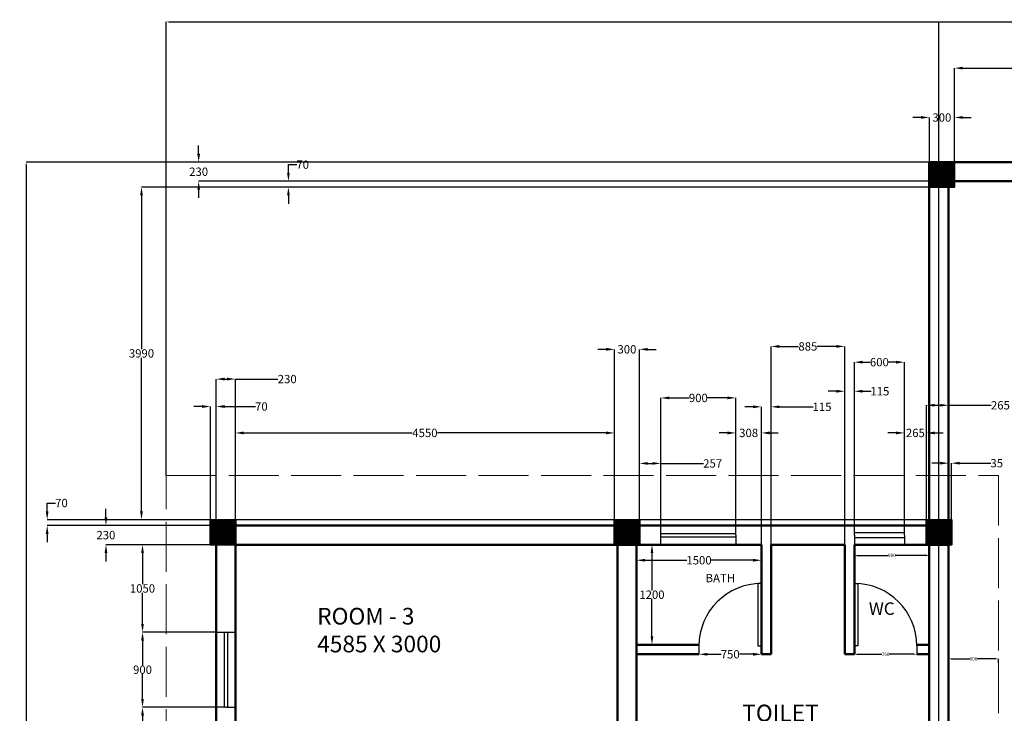
# Model space of a CAD drawing. Units: millimetres. Extents: x -17156 to 39375, y -45872 to -24892.
# Tile 3 of 12: x -17156 to -5337, y -33861 to -25539. Entities that reach past the tile are written whole.
import ezdxf

# ---------------------------------------------------------------- set-up
doc = ezdxf.new("R2010")
doc.units = ezdxf.units.MM
doc.header["$MEASUREMENT"] = 0
doc.linetypes.add('ACAD_ISO02W100', pattern=[15, 12, -3])
for name, color, linetype, lineweight in [('A-ANNO-DIMS', 2, 'Continuous', 18), ('A-AREA-IDEN', 4, 'Continuous', 25), ('A-COLS', 7, 'Continuous', 40), ('A-ROOF-OVHD', 8, 'ACAD_ISO02W100', 18), ('DOORS', 6, 'Continuous', 25), ('WALLS', 5, 'Continuous', 50), ('WINDOW', 240, 'Continuous', 25)]:
    doc.layers.add(name, color=color, linetype=linetype, lineweight=lineweight)
doc.styles.get("Standard").update_dxf_attribs({"font": 'arial.ttf'})
doc.dimstyles.get("Standard").update_dxf_attribs({"dimtxt": 40, "dimasz": 30.18, "dimexe": 0, "dimexo": 0.0625, "dimgap": 0.09, "dimtad": 0, "dimtih": 1, "dimtoh": 1, "dimdec": 0, "dimzin": 0, "dimdsep": 46, "dimtxsty": 'Standard', "dimcen": 0.09, "dimadec": 0, "dimazin": 0, "dimtfac": 1, "dimtdec": 0, "dimtofl": 0, "dimtmove": 0, "dimatfit": 3, "dimfxl": 1, "dimtolj": 1, "dimtzin": 0, "dimarcsym": 0})

# ---------------------------------------------------------------- blocks, each defined once
blk = doc.blocks.new('*U3')
for p, q in [((-750, 0), (-750, -100)), ((0, 0), (0, -100))]:
    blk.add_line(p, q)
blk.add_lwpolyline([(0, 0), (0, 750), (-43.75, 750), (-43.75, 0)], close=True)
blk.add_arc((0, 0), 750, 90, 180)
blk = doc.blocks.new('*U5')
for p, q in [((0, 0), (0, -100)), ((750, 0), (750, -100))]:
    blk.add_line(p, q)
blk.add_lwpolyline([(0, 0), (0, 750), (43.75, 750), (43.75, 0)], close=True)
blk.add_arc((0, 0), 750, 0, 90)
blk = doc.blocks.new('*D23')
at = {"layer": 'A-ANNO-DIMS', "color": 0, "lineweight": -2, "transparency": 16777216}
for p, q in [((-14797, -33788), (-15682, -33788)), ((-15682, -33888), (-15682, -34262)), ((-15682, -34738), (-15682, -34364)), ((-14867, -34838), (-15682, -34838))]:
    blk.add_line(p, q, dxfattribs=at)
at = {"layer": 'A-ANNO-DIMS', "color": 0, "lineweight": 100, "transparency": 16777216}
for points in [[(-15698, -33888), (-15665, -33888), (-15682, -33788)], [(-15698, -34738), (-15665, -34738), (-15682, -34838)]]:
    blk.add_solid(points, dxfattribs=at)
at = {"layer": 'Defpoints', "color": 0, "lineweight": 100, "transparency": 16777216}
for p in [(-15682, -33788), (-14797, -33788), (-14867, -34838)]:
    blk.add_point(p, dxfattribs=at)
at = {"layer": 'A-ANNO-DIMS', "color": 0, "transparency": 16777216, "insert": (-15682, -34313), "char_height": 100, "attachment_point": 5}
blk.add_mtext('\\A1;1050', dxfattribs=at)
blk = doc.blocks.new('*D24')
at = {"layer": 'A-ANNO-DIMS', "color": 0, "lineweight": -2, "transparency": 16777216}
for p, q in [((-14797, -32888), (-15682, -32888)), ((-15682, -32988), (-15682, -33287)), ((-15682, -33688), (-15682, -33389)), ((-14797, -33788), (-15682, -33788))]:
    blk.add_line(p, q, dxfattribs=at)
at = {"layer": 'A-ANNO-DIMS', "color": 0, "lineweight": 100, "transparency": 16777216}
for points in [[(-15698, -32988), (-15665, -32988), (-15682, -32888)], [(-15698, -33688), (-15665, -33688), (-15682, -33788)]]:
    blk.add_solid(points, dxfattribs=at)
at = {"layer": 'Defpoints', "color": 0, "lineweight": 100, "transparency": 16777216}
for p in [(-15682, -32888), (-14797, -32888), (-14797, -33788)]:
    blk.add_point(p, dxfattribs=at)
at = {"layer": 'A-ANNO-DIMS', "color": 0, "transparency": 16777216, "insert": (-15682, -33338), "char_height": 100, "attachment_point": 5}
blk.add_mtext('\\A1;900', dxfattribs=at)
blk = doc.blocks.new('*D25')
at = {"layer": 'A-ANNO-DIMS', "color": 0, "lineweight": -2, "transparency": 16777216}
for p, q in [((-14867, -31838), (-15682, -31838)), ((-15682, -31938), (-15682, -32312)), ((-15682, -32788), (-15682, -32414)), ((-14797, -32888), (-15682, -32888))]:
    blk.add_line(p, q, dxfattribs=at)
at = {"layer": 'A-ANNO-DIMS', "color": 0, "lineweight": 100, "transparency": 16777216}
for points in [[(-15698, -31938), (-15665, -31938), (-15682, -31838)], [(-15698, -32788), (-15665, -32788), (-15682, -32888)]]:
    blk.add_solid(points, dxfattribs=at)
at = {"layer": 'Defpoints', "color": 0, "lineweight": 100, "transparency": 16777216}
for p in [(-15682, -31838), (-14867, -31838), (-14797, -32888)]:
    blk.add_point(p, dxfattribs=at)
at = {"layer": 'A-ANNO-DIMS', "color": 0, "transparency": 16777216, "insert": (-15682, -32363), "char_height": 100, "attachment_point": 5}
blk.add_mtext('\\A1;1050', dxfattribs=at)
blk = doc.blocks.new('*D26')
at = {"layer": 'A-ANNO-DIMS', "color": 0, "lineweight": -2, "transparency": 16777216}
for p, q in [((-16121, -31508), (-16121, -31408)), ((-14797, -31608), (-16121, -31608)), ((-14867, -31838), (-16121, -31838)), ((-16121, -31938), (-16121, -32038))]:
    blk.add_line(p, q, dxfattribs=at)
at = {"layer": 'A-ANNO-DIMS', "color": 0, "lineweight": 100, "transparency": 16777216}
for points in [[(-16137, -31508), (-16104, -31508), (-16121, -31608)], [(-16137, -31938), (-16104, -31938), (-16121, -31838)]]:
    blk.add_solid(points, dxfattribs=at)
at = {"layer": 'Defpoints', "color": 0, "lineweight": 100, "transparency": 16777216}
for p in [(-16121, -31608), (-14797, -31608), (-14867, -31838)]:
    blk.add_point(p, dxfattribs=at)
at = {"layer": 'A-ANNO-DIMS', "color": 0, "transparency": 16777216, "insert": (-16121, -31723), "char_height": 100, "attachment_point": 5}
blk.add_mtext('\\A1;230', dxfattribs=at)
blk = doc.blocks.new('*D27')
at = {"layer": 'A-ANNO-DIMS', "color": 0, "lineweight": -2, "transparency": 16777216}
for p, q in [((-16826, -31438), (-16826, -31338)), ((-16826, -31338), (-16726, -31338)), ((-14867, -31538), (-16826, -31538)), ((-14797, -31608), (-16826, -31608)), ((-16826, -31708), (-16826, -31808))]:
    blk.add_line(p, q, dxfattribs=at)
at = {"layer": 'A-ANNO-DIMS', "color": 0, "lineweight": 100, "transparency": 16777216}
for points in [[(-16843, -31438), (-16810, -31438), (-16826, -31538)], [(-16843, -31708), (-16810, -31708), (-16826, -31608)]]:
    blk.add_solid(points, dxfattribs=at)
at = {"layer": 'Defpoints', "color": 0, "lineweight": 100, "transparency": 16777216}
for p in [(-16826, -31538), (-14867, -31538), (-14797, -31608)]:
    blk.add_point(p, dxfattribs=at)
at = {"layer": 'A-ANNO-DIMS', "color": 0, "transparency": 16777216, "insert": (-16655, -31338), "char_height": 100, "attachment_point": 5}
blk.add_mtext('\\A1;70', dxfattribs=at)
blk = doc.blocks.new('*D28')
at = {"layer": 'A-ANNO-DIMS', "color": 0, "lineweight": -2, "transparency": 16777216}
for p, q in [((-6237, -27548), (-15694, -27548)), ((-15694, -27648), (-15694, -29492)), ((-15694, -31438), (-15694, -29594)), ((-6272, -31538), (-15694, -31538))]:
    blk.add_line(p, q, dxfattribs=at)
at = {"layer": 'A-ANNO-DIMS', "color": 0, "lineweight": 100, "transparency": 16777216}
for points in [[(-15711, -27648), (-15677, -27648), (-15694, -27548)], [(-15711, -31438), (-15677, -31438), (-15694, -31538)]]:
    blk.add_solid(points, dxfattribs=at)
at = {"layer": 'Defpoints', "color": 0, "lineweight": 100, "transparency": 16777216}
for p in [(-15694, -27548), (-6237, -27548), (-6272, -31538)]:
    blk.add_point(p, dxfattribs=at)
at = {"layer": 'A-ANNO-DIMS', "color": 0, "transparency": 16777216, "insert": (-15694, -29543), "char_height": 100, "attachment_point": 5}
blk.add_mtext('\\A1;3990', dxfattribs=at)
blk = doc.blocks.new('*D29')
at = {"layer": 'A-ANNO-DIMS', "color": 0, "lineweight": -2, "transparency": 16777216}
for p, q in [((-13930, -27378), (-13930, -27278)), ((-13930, -27278), (-13830, -27278)), ((-6237, -27478), (-13930, -27478)), ((-6237, -27548), (-13930, -27548)), ((-13930, -27648), (-13930, -27748))]:
    blk.add_line(p, q, dxfattribs=at)
at = {"layer": 'A-ANNO-DIMS', "color": 0, "lineweight": 100, "transparency": 16777216}
for points in [[(-13947, -27378), (-13914, -27378), (-13930, -27478)], [(-13947, -27648), (-13914, -27648), (-13930, -27548)]]:
    blk.add_solid(points, dxfattribs=at)
at = {"layer": 'Defpoints', "color": 0, "lineweight": 100, "transparency": 16777216}
for p in [(-13930, -27478), (-6237, -27478), (-6237, -27548)]:
    blk.add_point(p, dxfattribs=at)
at = {"layer": 'A-ANNO-DIMS', "color": 0, "transparency": 16777216, "insert": (-13759, -27278), "char_height": 100, "attachment_point": 5}
blk.add_mtext('\\A1;70', dxfattribs=at)
blk = doc.blocks.new('*D30')
at = {"layer": 'A-ANNO-DIMS', "color": 0, "lineweight": -2, "transparency": 16777216}
for p, q in [((-15008, -27148), (-15008, -27048)), ((-6237, -27248), (-15008, -27248)), ((-6237, -27478), (-15008, -27478)), ((-15008, -27578), (-15008, -27678))]:
    blk.add_line(p, q, dxfattribs=at)
at = {"layer": 'A-ANNO-DIMS', "color": 0, "lineweight": 100, "transparency": 16777216}
for points in [[(-15024, -27148), (-14991, -27148), (-15008, -27248)], [(-15024, -27578), (-14991, -27578), (-15008, -27478)]]:
    blk.add_solid(points, dxfattribs=at)
at = {"layer": 'Defpoints', "color": 0, "lineweight": 100, "transparency": 16777216}
for p in [(-15008, -27248), (-6237, -27248), (-6237, -27478)]:
    blk.add_point(p, dxfattribs=at)
at = {"layer": 'A-ANNO-DIMS', "color": 0, "transparency": 16777216, "insert": (-15008, -27363), "char_height": 100, "attachment_point": 5}
blk.add_mtext('\\A1;230', dxfattribs=at)
blk = doc.blocks.new('*D52')
at = {"layer": 'A-ANNO-DIMS', "color": 0, "lineweight": -2, "transparency": 16777216}
for p, q in [((-14967, -30180), (-15067, -30180)), ((-14867, -31538), (-14867, -30180)), ((-14797, -31608), (-14797, -30180)), ((-14697, -30180), (-14326, -30180))]:
    blk.add_line(p, q, dxfattribs=at)
at = {"layer": 'A-ANNO-DIMS', "color": 0, "lineweight": 100, "transparency": 16777216}
for points in [[(-14967, -30163), (-14967, -30197), (-14867, -30180)], [(-14697, -30163), (-14697, -30197), (-14797, -30180)]]:
    blk.add_solid(points, dxfattribs=at)
at = {"layer": 'Defpoints', "color": 0, "lineweight": 100, "transparency": 16777216}
for p in [(-14797, -30180), (-14867, -31538), (-14797, -31608)]:
    blk.add_point(p, dxfattribs=at)
at = {"layer": 'A-ANNO-DIMS', "color": 0, "transparency": 16777216, "insert": (-14255, -30180), "char_height": 100, "attachment_point": 5}
blk.add_mtext('\\A1;70', dxfattribs=at)
blk = doc.blocks.new('*D53')
at = {"layer": 'A-ANNO-DIMS', "color": 0, "lineweight": -2, "transparency": 16777216}
for p, q in [((-14797, -31608), (-14797, -29851)), ((-14697, -29851), (-14667, -29851)), ((-14567, -31538), (-14567, -29851)), ((-14567, -29851), (-14056, -29851))]:
    blk.add_line(p, q, dxfattribs=at)
at = {"layer": 'A-ANNO-DIMS', "color": 0, "lineweight": 100, "transparency": 16777216}
for points in [[(-14697, -29834), (-14697, -29867), (-14797, -29851)], [(-14667, -29834), (-14667, -29867), (-14567, -29851)]]:
    blk.add_solid(points, dxfattribs=at)
at = {"layer": 'Defpoints', "color": 0, "lineweight": 100, "transparency": 16777216}
for p in [(-14567, -29851), (-14567, -31538), (-14797, -31608)]:
    blk.add_point(p, dxfattribs=at)
at = {"layer": 'A-ANNO-DIMS', "color": 0, "transparency": 16777216, "insert": (-13945, -29851), "char_height": 100, "attachment_point": 5}
blk.add_mtext('\\A1;230', dxfattribs=at)
blk = doc.blocks.new('*D54')
at = {"layer": 'A-ANNO-DIMS', "color": 0, "lineweight": -2, "transparency": 16777216}
for p, q in [((-14567, -31538), (-14567, -30497)), ((-14467, -30497), (-12444, -30497)), ((-10117, -30497), (-12141, -30497)), ((-10017, -31538), (-10017, -30497))]:
    blk.add_line(p, q, dxfattribs=at)
at = {"layer": 'A-ANNO-DIMS', "color": 0, "lineweight": 100, "transparency": 16777216}
for points in [[(-14467, -30480), (-14467, -30514), (-14567, -30497)], [(-10117, -30480), (-10117, -30514), (-10017, -30497)]]:
    blk.add_solid(points, dxfattribs=at)
at = {"layer": 'Defpoints', "color": 0, "lineweight": 100, "transparency": 16777216}
for p in [(-10017, -30497), (-14567, -31538), (-10017, -31538)]:
    blk.add_point(p, dxfattribs=at)
at = {"layer": 'A-ANNO-DIMS', "color": 0, "transparency": 16777216, "insert": (-12292, -30497), "char_height": 100, "attachment_point": 5}
blk.add_mtext('\\A1;4550', dxfattribs=at)
blk = doc.blocks.new('*D55')
at = {"layer": 'A-ANNO-DIMS', "color": 0, "lineweight": -2, "transparency": 16777216}
for p, q in [((-10117, -29494), (-10217, -29494)), ((-10017, -31538), (-10017, -29494)), ((-9717, -31538), (-9717, -29494)), ((-9617, -29494), (-9517, -29494))]:
    blk.add_line(p, q, dxfattribs=at)
at = {"layer": 'A-ANNO-DIMS', "color": 0, "lineweight": 100, "transparency": 16777216}
for points in [[(-10117, -29477), (-10117, -29511), (-10017, -29494)], [(-9617, -29477), (-9617, -29511), (-9717, -29494)]]:
    blk.add_solid(points, dxfattribs=at)
at = {"layer": 'Defpoints', "color": 0, "lineweight": 100, "transparency": 16777216}
for p in [(-9717, -29494), (-10017, -31538), (-9717, -31538)]:
    blk.add_point(p, dxfattribs=at)
at = {"layer": 'A-ANNO-DIMS', "color": 0, "transparency": 16777216, "insert": (-9867, -29494), "char_height": 100, "attachment_point": 5}
blk.add_mtext('\\A1;300', dxfattribs=at)
blk = doc.blocks.new('*D56')
at = {"layer": 'A-ANNO-DIMS', "color": 0, "lineweight": -2, "transparency": 16777216}
for p, q in [((-9717, -31538), (-9717, -30863)), ((-9617, -30863), (-9560, -30863)), ((-9460, -31608), (-9460, -30863)), ((-9460, -30863), (-8949, -30863))]:
    blk.add_line(p, q, dxfattribs=at)
at = {"layer": 'A-ANNO-DIMS', "color": 0, "lineweight": 100, "transparency": 16777216}
for points in [[(-9617, -30846), (-9617, -30879), (-9717, -30863)], [(-9560, -30846), (-9560, -30879), (-9460, -30863)]]:
    blk.add_solid(points, dxfattribs=at)
at = {"layer": 'Defpoints', "color": 0, "lineweight": 100, "transparency": 16777216}
for p in [(-9460, -30863), (-9717, -31538), (-9460, -31608)]:
    blk.add_point(p, dxfattribs=at)
at = {"layer": 'A-ANNO-DIMS', "color": 0, "transparency": 16777216, "insert": (-8838, -30863), "char_height": 100, "attachment_point": 5}
blk.add_mtext('\\A1;257', dxfattribs=at)
blk = doc.blocks.new('*D57')
at = {"layer": 'A-ANNO-DIMS', "color": 0, "lineweight": -2, "transparency": 16777216}
for p, q in [((-9460, -31608), (-9460, -30077)), ((-9360, -30077), (-9121, -30077)), ((-8660, -30077), (-8900, -30077)), ((-8560, -31608), (-8560, -30077))]:
    blk.add_line(p, q, dxfattribs=at)
at = {"layer": 'A-ANNO-DIMS', "color": 0, "lineweight": 100, "transparency": 16777216}
for points in [[(-9360, -30060), (-9360, -30093), (-9460, -30077)], [(-8660, -30060), (-8660, -30093), (-8560, -30077)]]:
    blk.add_solid(points, dxfattribs=at)
at = {"layer": 'Defpoints', "color": 0, "lineweight": 100, "transparency": 16777216}
for p in [(-8560, -30077), (-9460, -31608), (-8560, -31608)]:
    blk.add_point(p, dxfattribs=at)
at = {"layer": 'A-ANNO-DIMS', "color": 0, "transparency": 16777216, "insert": (-9010, -30077), "char_height": 100, "attachment_point": 5}
blk.add_mtext('\\A1;900', dxfattribs=at)
blk = doc.blocks.new('*D58')
at = {"layer": 'A-ANNO-DIMS', "color": 0, "lineweight": -2, "transparency": 16777216}
for p, q in [((-8660, -30497), (-8760, -30497)), ((-8560, -31608), (-8560, -30497)), ((-8252, -31838), (-8252, -30497)), ((-8152, -30497), (-8052, -30497))]:
    blk.add_line(p, q, dxfattribs=at)
at = {"layer": 'A-ANNO-DIMS', "color": 0, "lineweight": 100, "transparency": 16777216}
for points in [[(-8660, -30480), (-8660, -30514), (-8560, -30497)], [(-8152, -30480), (-8152, -30514), (-8252, -30497)]]:
    blk.add_solid(points, dxfattribs=at)
at = {"layer": 'Defpoints', "color": 0, "lineweight": 100, "transparency": 16777216}
for p in [(-8252, -30497), (-8560, -31608), (-8252, -31838)]:
    blk.add_point(p, dxfattribs=at)
at = {"layer": 'A-ANNO-DIMS', "color": 0, "transparency": 16777216, "insert": (-8406, -30497), "char_height": 100, "attachment_point": 5}
blk.add_mtext('\\A1;308', dxfattribs=at)
blk = doc.blocks.new('*D59')
at = {"layer": 'A-ANNO-DIMS', "color": 0, "lineweight": -2, "transparency": 16777216}
for p, q in [((-8352, -30184), (-8452, -30184)), ((-8252, -31838), (-8252, -30184)), ((-8137, -31838), (-8137, -30184)), ((-8037, -30184), (-7631, -30184))]:
    blk.add_line(p, q, dxfattribs=at)
at = {"layer": 'A-ANNO-DIMS', "color": 0, "lineweight": 100, "transparency": 16777216}
for points in [[(-8352, -30167), (-8352, -30200), (-8252, -30184)], [(-8037, -30167), (-8037, -30200), (-8137, -30184)]]:
    blk.add_solid(points, dxfattribs=at)
at = {"layer": 'Defpoints', "color": 0, "lineweight": 100, "transparency": 16777216}
for p in [(-8137, -30184), (-8252, -31838), (-8137, -31838)]:
    blk.add_point(p, dxfattribs=at)
at = {"layer": 'A-ANNO-DIMS', "color": 0, "transparency": 16777216, "insert": (-7525, -30184), "char_height": 100, "attachment_point": 5}
blk.add_mtext('\\A1;115', dxfattribs=at)
blk = doc.blocks.new('*D60')
at = {"layer": 'A-ANNO-DIMS', "color": 0, "lineweight": -2, "transparency": 16777216}
for p, q in [((-8137, -31838), (-8137, -29459)), ((-8037, -29459), (-7806, -29459)), ((-7352, -29459), (-7584, -29459)), ((-7252, -31838), (-7252, -29459))]:
    blk.add_line(p, q, dxfattribs=at)
at = {"layer": 'A-ANNO-DIMS', "color": 0, "lineweight": 100, "transparency": 16777216}
for points in [[(-8037, -29442), (-8037, -29476), (-8137, -29459)], [(-7352, -29442), (-7352, -29476), (-7252, -29459)]]:
    blk.add_solid(points, dxfattribs=at)
at = {"layer": 'Defpoints', "color": 0, "lineweight": 100, "transparency": 16777216}
for p in [(-7252, -29459), (-8137, -31838), (-7252, -31838)]:
    blk.add_point(p, dxfattribs=at)
at = {"layer": 'A-ANNO-DIMS', "color": 0, "transparency": 16777216, "insert": (-7695, -29459), "char_height": 100, "attachment_point": 5}
blk.add_mtext('\\A1;885', dxfattribs=at)
blk = doc.blocks.new('*D61')
at = {"layer": 'A-ANNO-DIMS', "color": 0, "lineweight": -2, "transparency": 16777216}
for p, q in [((-7352, -29997), (-7452, -29997)), ((-7252, -31838), (-7252, -29997)), ((-7137, -31608), (-7137, -29997)), ((-7037, -29997), (-6937, -29997))]:
    blk.add_line(p, q, dxfattribs=at)
at = {"layer": 'A-ANNO-DIMS', "color": 0, "lineweight": 100, "transparency": 16777216}
for points in [[(-7352, -29980), (-7352, -30014), (-7252, -29997)], [(-7037, -29980), (-7037, -30014), (-7137, -29997)]]:
    blk.add_solid(points, dxfattribs=at)
at = {"layer": 'Defpoints', "color": 0, "lineweight": 100, "transparency": 16777216}
for p in [(-7137, -29997), (-7137, -31608), (-7252, -31838)]:
    blk.add_point(p, dxfattribs=at)
at = {"layer": 'A-ANNO-DIMS', "color": 0, "transparency": 16777216, "insert": (-6831, -29997), "char_height": 100, "attachment_point": 5}
blk.add_mtext('\\A1;115', dxfattribs=at)
blk = doc.blocks.new('*D62')
at = {"layer": 'A-ANNO-DIMS', "color": 0, "lineweight": -2, "transparency": 16777216}
for p, q in [((-7137, -31608), (-7137, -29648)), ((-7037, -29648), (-6948, -29648)), ((-6637, -29648), (-6727, -29648)), ((-6537, -31608), (-6537, -29648))]:
    blk.add_line(p, q, dxfattribs=at)
at = {"layer": 'A-ANNO-DIMS', "color": 0, "lineweight": 100, "transparency": 16777216}
for points in [[(-7037, -29631), (-7037, -29665), (-7137, -29648)], [(-6637, -29631), (-6637, -29665), (-6537, -29648)]]:
    blk.add_solid(points, dxfattribs=at)
at = {"layer": 'Defpoints', "color": 0, "lineweight": 100, "transparency": 16777216}
for p in [(-6537, -29648), (-7137, -31608), (-6537, -31608)]:
    blk.add_point(p, dxfattribs=at)
at = {"layer": 'A-ANNO-DIMS', "color": 0, "transparency": 16777216, "insert": (-6837, -29648), "char_height": 100, "attachment_point": 5}
blk.add_mtext('\\A1;600', dxfattribs=at)
blk = doc.blocks.new('*D63')
at = {"layer": 'A-ANNO-DIMS', "color": 0, "lineweight": -2, "transparency": 16777216}
for p, q in [((-6637, -30497), (-6737, -30497)), ((-6537, -31608), (-6537, -30497)), ((-6272, -31538), (-6272, -30497)), ((-6172, -30497), (-6072, -30497))]:
    blk.add_line(p, q, dxfattribs=at)
at = {"layer": 'A-ANNO-DIMS', "color": 0, "lineweight": 100, "transparency": 16777216}
for points in [[(-6637, -30480), (-6637, -30514), (-6537, -30497)], [(-6172, -30480), (-6172, -30514), (-6272, -30497)]]:
    blk.add_solid(points, dxfattribs=at)
at = {"layer": 'Defpoints', "color": 0, "lineweight": 100, "transparency": 16777216}
for p in [(-6272, -30497), (-6272, -31538), (-6537, -31608)]:
    blk.add_point(p, dxfattribs=at)
at = {"layer": 'A-ANNO-DIMS', "color": 0, "transparency": 16777216, "insert": (-6405, -30497), "char_height": 100, "attachment_point": 5}
blk.add_mtext('\\A1;265', dxfattribs=at)
blk = doc.blocks.new('*D64')
at = {"layer": 'A-ANNO-DIMS', "color": 0, "lineweight": -2, "transparency": 16777216}
for p, q in [((-6272, -31538), (-6272, -30165)), ((-6172, -30165), (-6107, -30165)), ((-6007, -31608), (-6007, -30165)), ((-6007, -30165), (-5496, -30165))]:
    blk.add_line(p, q, dxfattribs=at)
at = {"layer": 'A-ANNO-DIMS', "color": 0, "lineweight": 100, "transparency": 16777216}
for points in [[(-6172, -30148), (-6172, -30181), (-6272, -30165)], [(-6107, -30148), (-6107, -30181), (-6007, -30165)]]:
    blk.add_solid(points, dxfattribs=at)
at = {"layer": 'Defpoints', "color": 0, "lineweight": 100, "transparency": 16777216}
for p in [(-6007, -30165), (-6272, -31538), (-6007, -31608)]:
    blk.add_point(p, dxfattribs=at)
at = {"layer": 'A-ANNO-DIMS', "color": 0, "transparency": 16777216, "insert": (-5384, -30165), "char_height": 100, "attachment_point": 5}
blk.add_mtext('\\A1;265', dxfattribs=at)
blk = doc.blocks.new('*D65')
at = {"layer": 'A-ANNO-DIMS', "color": 0, "lineweight": -2, "transparency": 16777216}
for p, q in [((-6107, -30860), (-6207, -30860)), ((-6007, -31608), (-6007, -30860)), ((-5972, -31538), (-5972, -30860)), ((-5872, -30860), (-5500, -30860))]:
    blk.add_line(p, q, dxfattribs=at)
at = {"layer": 'A-ANNO-DIMS', "color": 0, "lineweight": 100, "transparency": 16777216}
for points in [[(-6107, -30843), (-6107, -30877), (-6007, -30860)], [(-5872, -30843), (-5872, -30877), (-5972, -30860)]]:
    blk.add_solid(points, dxfattribs=at)
at = {"layer": 'Defpoints', "color": 0, "lineweight": 100, "transparency": 16777216}
for p in [(-5972, -30860), (-5972, -31538), (-6007, -31608)]:
    blk.add_point(p, dxfattribs=at)
at = {"layer": 'A-ANNO-DIMS', "color": 0, "transparency": 16777216, "insert": (-5428, -30860), "char_height": 100, "attachment_point": 5}
blk.add_mtext('\\A1;35', dxfattribs=at)
blk = doc.blocks.new('*D66')
at = {"layer": 'A-ANNO-DIMS', "color": 0, "lineweight": -2, "transparency": 16777216}
for p, q in [((-6337, -26712), (-6437, -26712)), ((-6237, -27248), (-6237, -26712)), ((-5937, -27248), (-5937, -26712)), ((-5837, -26712), (-5737, -26712))]:
    blk.add_line(p, q, dxfattribs=at)
at = {"layer": 'A-ANNO-DIMS', "color": 0, "lineweight": 100, "transparency": 16777216}
for points in [[(-6337, -26695), (-6337, -26728), (-6237, -26712)], [(-5837, -26695), (-5837, -26728), (-5937, -26712)]]:
    blk.add_solid(points, dxfattribs=at)
at = {"layer": 'Defpoints', "color": 0, "lineweight": 100, "transparency": 16777216}
for p in [(-5937, -26712), (-6237, -27248), (-5937, -27248)]:
    blk.add_point(p, dxfattribs=at)
at = {"layer": 'A-ANNO-DIMS', "color": 0, "transparency": 16777216, "insert": (-6087, -26712), "char_height": 100, "attachment_point": 5}
blk.add_mtext('\\A1;300', dxfattribs=at)
blk = doc.blocks.new('*D67')
at = {"layer": 'A-ANNO-DIMS', "color": 0, "lineweight": -2, "transparency": 16777216}
for p, q in [((-5937, -27248), (-5937, -26120)), ((-5837, -26120), (-4007, -26120)), ((-1872, -26120), (-3703, -26120)), ((-1772, -27248), (-1772, -26120))]:
    blk.add_line(p, q, dxfattribs=at)
at = {"layer": 'A-ANNO-DIMS', "color": 0, "lineweight": 100, "transparency": 16777216}
for points in [[(-5837, -26103), (-5837, -26136), (-5937, -26120)], [(-1872, -26103), (-1872, -26136), (-1772, -26120)]]:
    blk.add_solid(points, dxfattribs=at)
at = {"layer": 'Defpoints', "color": 0, "lineweight": 100, "transparency": 16777216}
for p in [(-1772, -26120), (-5937, -27248), (-1772, -27248)]:
    blk.add_point(p, dxfattribs=at)
at = {"layer": 'A-ANNO-DIMS', "color": 0, "transparency": 16777216, "insert": (-3855, -26120), "char_height": 100, "attachment_point": 5}
blk.add_mtext('\\A1;4165', dxfattribs=at)
blk = doc.blocks.new('*D77')
at = {"layer": 'A-ANNO-DIMS', "color": 0, "lineweight": -2, "transparency": 16777216}
for p, q in [((-9327, -31838), (-9567, -31838)), ((-9567, -31938), (-9567, -32387)), ((-9567, -32938), (-9567, -32489)), ((-9377, -33038), (-9567, -33038))]:
    blk.add_line(p, q, dxfattribs=at)
at = {"layer": 'A-ANNO-DIMS', "color": 0, "lineweight": 100, "transparency": 16777216}
for points in [[(-9583, -31938), (-9550, -31938), (-9567, -31838)], [(-9583, -32938), (-9550, -32938), (-9567, -33038)]]:
    blk.add_solid(points, dxfattribs=at)
at = {"layer": 'Defpoints', "color": 0, "lineweight": 100, "transparency": 16777216}
for p in [(-9327, -31838), (-9567, -33038), (-9377, -33038)]:
    blk.add_point(p, dxfattribs=at)
at = {"layer": 'A-ANNO-DIMS', "color": 0, "transparency": 16777216, "insert": (-9567, -32438), "char_height": 100, "attachment_point": 5}
blk.add_mtext('\\A1;1200', dxfattribs=at)
blk = doc.blocks.new('*D78')
at = {"layer": 'A-ANNO-DIMS', "color": 0, "lineweight": -2, "transparency": 16777216}
for p, q in [((-9752, -31957), (-9752, -32025)), ((-9652, -32025), (-9147, -32025)), ((-8352, -32025), (-8858, -32025)), ((-8252, -31957), (-8252, -32025))]:
    blk.add_line(p, q, dxfattribs=at)
at = {"layer": 'A-ANNO-DIMS', "color": 0, "lineweight": 100, "transparency": 16777216}
for points in [[(-9652, -32008), (-9652, -32041), (-9752, -32025)], [(-8352, -32008), (-8352, -32041), (-8252, -32025)]]:
    blk.add_solid(points, dxfattribs=at)
at = {"layer": 'Defpoints', "color": 0, "lineweight": 100, "transparency": 16777216}
for p in [(-9752, -31957), (-9752, -32025), (-8252, -31957)]:
    blk.add_point(p, dxfattribs=at)
at = {"layer": 'A-ANNO-DIMS', "color": 0, "transparency": 16777216, "insert": (-9002, -32025), "char_height": 100, "attachment_point": 5}
blk.add_mtext('\\A1;1500', dxfattribs=at)
blk = doc.blocks.new('*D79')
at = {"layer": 'A-ANNO-DIMS', "color": 0, "lineweight": -2, "transparency": 16777216}
for p, q in [((-9002, -33153), (-9002, -33153)), ((-8902, -33153), (-8737, -33153)), ((-8352, -33153), (-8517, -33153)), ((-8252, -33153), (-8252, -33153))]:
    blk.add_line(p, q, dxfattribs=at)
at = {"layer": 'A-ANNO-DIMS', "color": 0, "lineweight": 100, "transparency": 16777216}
for points in [[(-8902, -33136), (-8902, -33170), (-9002, -33153)], [(-8352, -33136), (-8352, -33170), (-8252, -33153)]]:
    blk.add_solid(points, dxfattribs=at)
at = {"layer": 'Defpoints', "color": 0, "lineweight": 100, "transparency": 16777216}
for p in [(-9002, -33153), (-8252, -33153), (-8252, -33153)]:
    blk.add_point(p, dxfattribs=at)
at = {"layer": 'A-ANNO-DIMS', "color": 0, "transparency": 16777216, "insert": (-8627, -33153), "char_height": 100, "attachment_point": 5}
blk.add_mtext('\\A1;750', dxfattribs=at)
blk = doc.blocks.new('*D80')
at = {"layer": 'A-ANNO-DIMS', "color": 0, "lineweight": -2, "transparency": 16777216}
for p, q in [((-7137, -33153), (-7137, -33153)), ((-7107, -33153), (-6806, -33153)), ((-6418, -33153), (-6718, -33153)), ((-6387, -33153), (-6387, -33153))]:
    blk.add_line(p, q, dxfattribs=at)
at = {"layer": 'A-ANNO-DIMS', "color": 0, "lineweight": 100, "transparency": 16777216}
for points in [[(-7107, -33148), (-7107, -33158), (-7137, -33153)], [(-6418, -33148), (-6418, -33158), (-6387, -33153)]]:
    blk.add_solid(points, dxfattribs=at)
at = {"layer": 'Defpoints', "color": 0, "lineweight": 100, "transparency": 16777216}
for p in [(-7137, -33153), (-6387, -33153), (-6387, -33153)]:
    blk.add_point(p, dxfattribs=at)
at = {"layer": 'A-ANNO-DIMS', "color": 0, "transparency": 16777216, "insert": (-6762, -33153), "char_height": 40, "attachment_point": 5}
blk.add_mtext('\\A1;750', dxfattribs=at)
blk = doc.blocks.new('*D81')
at = {"layer": 'A-ANNO-DIMS', "color": 0, "lineweight": -2, "transparency": 16777216}
for p, q in [((-7137, -32025), (-7137, -31966)), ((-7107, -31966), (-6732, -31966)), ((-6268, -31966), (-6643, -31966)), ((-6237, -32025), (-6237, -31966))]:
    blk.add_line(p, q, dxfattribs=at)
at = {"layer": 'A-ANNO-DIMS', "color": 0, "lineweight": 100, "transparency": 16777216}
for points in [[(-7107, -31961), (-7107, -31971), (-7137, -31966)], [(-6268, -31961), (-6268, -31971), (-6237, -31966)]]:
    blk.add_solid(points, dxfattribs=at)
at = {"layer": 'Defpoints', "color": 0, "lineweight": 100, "transparency": 16777216}
for p in [(-7137, -32025), (-6237, -31966), (-6237, -32025)]:
    blk.add_point(p, dxfattribs=at)
at = {"layer": 'A-ANNO-DIMS', "color": 0, "transparency": 16777216, "insert": (-6687, -31966), "char_height": 40, "attachment_point": 5}
blk.add_mtext('\\A1;900', dxfattribs=at)
blk = doc.blocks.new('*D111')
at = {"layer": 'A-ANNO-DIMS', "color": 0, "lineweight": -2, "transparency": 16777216}
for p, q in [((-6007, -33257), (-6007, -33208)), ((-5977, -33208), (-5752, -33208)), ((-5438, -33208), (-5663, -33208)), ((-5407, -33257), (-5407, -33208))]:
    blk.add_line(p, q, dxfattribs=at)
at = {"layer": 'A-ANNO-DIMS', "color": 0, "lineweight": 100, "transparency": 16777216}
for points in [[(-5977, -33203), (-5977, -33213), (-6007, -33208)], [(-5438, -33203), (-5438, -33213), (-5407, -33208)]]:
    blk.add_solid(points, dxfattribs=at)
at = {"layer": 'Defpoints', "color": 0, "lineweight": 100, "transparency": 16777216}
for p in [(-6007, -33208), (-6007, -33257), (-5407, -33257)]:
    blk.add_point(p, dxfattribs=at)
at = {"layer": 'A-ANNO-DIMS', "color": 0, "transparency": 16777216, "insert": (-5707, -33208), "char_height": 40, "attachment_point": 5}
blk.add_mtext('\\A1;600', dxfattribs=at)
blk = doc.blocks.new('WIN-900x230')
for p, q in [((0, 900), (230, 900)), ((95, 900), (95, 0)), ((135, 900), (135, 0)), ((115, 0), (0, 0)), ((115, 0), (230, 0))]:
    blk.add_line(p, q)
blk = doc.blocks.new('COL-300x300')
h = blk.add_hatch()
h.set_pattern_fill('ANSI31', color=256)
h.paths.add_polyline_path([(300, 300), (0, 300), (0, 0), (300, 0)])
blk.add_lwpolyline([(0, 300), (300, 300), (300, 0), (0, 0)], close=True)
blk = doc.blocks.new('*D144')
at = {"layer": 'A-ANNO-DIMS', "color": 0, "lineweight": -2, "transparency": 16777216}
for p, q in [((-15397, -31008), (-15397, -25565)), ((-15367, -25565), (-1063, -25565)), ((13392, -25565), (-912, -25565)), ((13423, -31008), (13423, -25565))]:
    blk.add_line(p, q, dxfattribs=at)
at = {"layer": 'A-ANNO-DIMS', "color": 0, "lineweight": 100, "transparency": 16777216}
for points in [[(-15367, -25560), (-15367, -25570), (-15397, -25565)], [(13392, -25560), (13392, -25570), (13423, -25565)]]:
    blk.add_solid(points, dxfattribs=at)
at = {"layer": 'Defpoints', "color": 0, "lineweight": 100, "transparency": 16777216}
for p in [(13423, -25565), (-15397, -31008), (13423, -31008)]:
    blk.add_point(p, dxfattribs=at)
at = {"layer": 'A-ANNO-DIMS', "color": 0, "transparency": 16777216, "insert": (-987, -25565), "char_height": 40, "attachment_point": 5}
blk.add_mtext('\\A1;28820', dxfattribs=at)
blk = doc.blocks.new('*D145')
at = {"layer": 'A-ANNO-DIMS', "color": 0, "lineweight": -2, "transparency": 16777216}
for p, q in [((-6237, -27248), (-17080, -27248)), ((-17080, -27278), (-17080, -35685)), ((-17080, -44133), (-17080, -35726)), ((-2887, -44163), (-17080, -44163))]:
    blk.add_line(p, q, dxfattribs=at)
at = {"layer": 'A-ANNO-DIMS', "color": 0, "lineweight": 100, "transparency": 16777216}
for points in [[(-17085, -27278), (-17075, -27278), (-17080, -27248)], [(-17085, -44133), (-17075, -44133), (-17080, -44163)]]:
    blk.add_solid(points, dxfattribs=at)
at = {"layer": 'Defpoints', "color": 0, "lineweight": 100, "transparency": 16777216}
for p in [(-6237, -27248), (-17080, -44163), (-2887, -44163)]:
    blk.add_point(p, dxfattribs=at)
at = {"layer": 'A-ANNO-DIMS', "color": 0, "transparency": 16777216, "insert": (-17080, -35705), "char_height": 40, "attachment_point": 5}
blk.add_mtext('\\A1;16915', dxfattribs=at)
blk = doc.blocks.new('*D151')
at = {"layer": 'A-ANNO-DIMS', "color": 0, "lineweight": -2, "transparency": 16777216}
for p, q in [((-6122, -42548), (-6122, -25565)), ((-6092, -25565), (-4413, -25565)), ((-2615, -25565), (-4294, -25565)), ((-2584, -42548), (-2584, -25565))]:
    blk.add_line(p, q, dxfattribs=at)
at = {"layer": 'A-ANNO-DIMS', "color": 0, "lineweight": 100, "transparency": 16777216}
for points in [[(-6092, -25560), (-6092, -25570), (-6122, -25565)], [(-2615, -25560), (-2615, -25570), (-2584, -25565)]]:
    blk.add_solid(points, dxfattribs=at)
at = {"layer": 'Defpoints', "color": 0, "lineweight": 100, "transparency": 16777216}
for p in [(-2584, -25565), (-6122, -42548), (-2584, -42548)]:
    blk.add_point(p, dxfattribs=at)
at = {"layer": 'A-ANNO-DIMS', "color": 0, "transparency": 16777216, "insert": (-4353, -25565), "char_height": 40, "attachment_point": 5}
blk.add_mtext('\\A1;3538', dxfattribs=at)

msp = doc.modelspace()

# ---------------------------------------------------------------- linework, layer by layer
at = {"layer": 'A-ROOF-OVHD', "ltscale": 50}
for p, q in [((-15397.35, -42662.85), (-15397.35, -31007.85)), ((-15397.35, -31007.85), (-5407.35, -31007.85)), ((-5407.35, -31007.85), (-5407.35, -34237.85))]:
    msp.add_line(p, q, dxfattribs=at)
at = {"layer": 'WALLS'}
for p, q in [((-6237.35, -27247.85), (-6237.35, -33152.85)), ((-6237.35, -27247.85), (-1472.35, -27247.85)), ((-6007.35, -27247.85), (-6007.35, -40562.85)), ((-6237.35, -27477.85), (-1472.35, -27477.85)), ((-14797.35, -42662.85), (-14797.35, -31607.85)), ((-14797.35, -31607.85), (-6007.35, -31607.85)), ((-9982.35, -35067.85), (-9982.35, -31607.85)), ((-9752.35, -35067.85), (-9752.35, -31607.85)), ((-14567.35, -31837.85), (-8252.35, -31837.85)), ((-14567.35, -34837.85), (-14567.35, -31837.85)), ((-8252.35, -33152.85), (-8252.35, -31837.85)), ((-8137.35, -33152.85), (-8137.35, -31837.85)), ((-8137.35, -31837.85), (-7252.35, -31837.85)), ((-7252.35, -31837.85), (-7252.35, -33152.85)), ((-7137.35, -31837.85), (-7137.35, -33152.85)), ((-7137.35, -31837.85), (-6007.35, -31837.85)), ((-9752.35, -33037.85), (-9002.2, -33037.85)), ((-6387.5, -33037.85), (-6237.35, -33037.85)), ((-9752.35, -33152.85), (-9002.35, -33152.85)), ((-8252.35, -33152.85), (-8137.35, -33152.85)), ((-7252.35, -33152.85), (-7137.35, -33152.85)), ((-6387.35, -33152.85), (-6237.35, -33152.85)), ((-6237.35, -33152.85), (-6237.35, -40562.85))]:
    msp.add_line(p, q, dxfattribs=at)
at = {"layer": 'WINDOW'}
for p, q in [((-7137.35, -31722.85), (-7137.35, -31607.85)), ((-6537.35, -31722.85), (-6537.35, -31607.85)), ((-7137.35, -31692.85), (-6537.35, -31692.85)), ((-7137.35, -31722.85), (-7137.35, -31837.85)), ((-7137.35, -31752.85), (-6537.35, -31752.85)), ((-6537.35, -31722.85), (-6537.35, -31837.85))]:
    msp.add_line(p, q, dxfattribs=at)

# ---------------------------------------------------------------- block references
at = {"layer": 'A-COLS'}
for p in [(-6237.35, -27547.85), (-6237.35, -27547.85), (-14867.35, -31837.85), (-10017.35, -31837.85), (-6272.35, -31837.85)]:
    msp.add_blockref('COL-300x300', p, dxfattribs=at)
at = {"layer": 'DOORS'}
for name, p in [('*U3', (-8252.35, -33052.85)), ('*U5', (-7137.35, -33052.85))]:
    msp.add_blockref(name, p, dxfattribs=at)
at = {"layer": 'WINDOW', "rotation": 89.99999999999984}
msp.add_blockref('WIN-900x230', (-8560.32, -31837.85), dxfattribs=at)
at = {"layer": 'WINDOW'}
msp.add_blockref('WIN-900x230', (-14797.35, -33788.06), dxfattribs=at)

# ---------------------------------------------------------------- texts
at = {"layer": 'A-AREA-IDEN', "attachment_point": 1}
for s, width, insert, char_height in [('{BATH }', 478.9193, (-8922.8, -32188.23), 100), ('{ROOM - 3\\P4585 X 3000}', 2531.4141, (-13585.33, -32596.36), 200), ('{WC}', 188.4214, (-6963.46, -32530.07), 150), ('{TOILET \\P3515 X 3000}', 1569.8583, (-8483.16, -33757.73), 200)]:
    msp.add_mtext_dynamic_manual_height_columns(s, width=width, gutter_width=1, heights=[0], dxfattribs=dict(at, insert=insert, char_height=char_height))

# ---------------------------------------------------------------- dimensions: what is measured, and where the dimension line sits
at = {"layer": 'A-ANNO-DIMS'}
for base, p1, p2, override, picture, middle in [((13422.65, -25564.85), (-15397.35, -31007.85), (13422.65, -31007.85), {"dimdec": 0, "dimlfac": 1, "dimrnd": 0, "dimzin": 0, "dimdsep": 46, "dimlunit": 2}, '*D144', (-987.35, -25564.85)), ((-2584.35, -25564.85), (-6122.35, -42547.85), (-2584.35, -42547.85), {"dimdec": 0, "dimlfac": 1, "dimrnd": 0, "dimzin": 0, "dimdsep": 46, "dimlunit": 2}, '*D151', (-4353.35, -25564.85)), ((-5937.35, -26711.58), (-6237.35, -27247.85), (-5937.35, -27247.85), {"dimtxt": 100, "dimasz": 100, "dimclrd": 0, "dimclre": 0, "dimclrt": 0}, '*D66', (-6087.35, -26711.58)), ((-9717.35, -29494.12), (-10017.35, -31537.85), (-9717.35, -31537.85), {"dimtxt": 100, "dimasz": 100, "dimclrd": 0, "dimclre": 0, "dimclrt": 0}, '*D55', (-9867.35, -29494.12)), ((-7252.35, -29458.89), (-8137.35, -31837.85), (-7252.35, -31837.85), {"dimtxt": 100, "dimasz": 100, "dimclrd": 0, "dimclre": 0, "dimclrt": 0}, '*D60', (-7694.85, -29458.89)), ((-7137.35, -29997.02), (-7252.35, -31837.85), (-7137.35, -31607.85), {"dimtxt": 100, "dimasz": 100, "dimclrd": 0, "dimclre": 0, "dimclrt": 0}, '*D61', (-6831.12, -29997.02)), ((-10017.35, -30496.87), (-14567.35, -31537.85), (-10017.35, -31537.85), {"dimtxt": 100, "dimasz": 100, "dimclrd": 0, "dimclre": 0, "dimclrt": 0}, '*D54', (-12292.35, -30496.87)), ((-8252.35, -30496.87), (-8560.32, -31607.85), (-8252.35, -31837.85), {"dimtxt": 100, "dimasz": 100, "dimclrd": 0, "dimclre": 0, "dimclrt": 0}, '*D58', (-8406.34, -30496.87)), ((-6272.35, -30496.87), (-6537.35, -31607.85), (-6272.35, -31537.85), {"dimtxt": 100, "dimasz": 100, "dimclrd": 0, "dimclre": 0, "dimclrt": 0}, '*D63', (-6404.85, -30496.87)), ((-9752.35, -32024.82), (-8252.35, -31956.53), (-9752.35, -31956.53), {"dimtxt": 100, "dimasz": 100, "dimclrd": 0, "dimclre": 0, "dimclrt": 0}, '*D78', (-9002.35, -32024.82)), ((-6237.35, -31965.73), (-7137.35, -32025.36), (-6237.35, -32025.36), {"dimclrd": 0, "dimclre": 0, "dimclrt": 0}, '*D81', (-6687.35, -31965.73)), ((-8252.35, -33152.85), (-9002.35, -33152.85), (-8252.35, -33152.85), {"dimtxt": 100, "dimasz": 100, "dimclrd": 0, "dimclre": 0, "dimclrt": 0}, '*D79', (-8627.35, -33152.85)), ((-6387.35, -33152.85), (-7137.35, -33152.85), (-6387.35, -33152.85), {"dimclrd": 0, "dimclre": 0, "dimclrt": 0}, '*D80', (-6762.35, -33152.85)), ((-6007.35, -33208.45), (-5407.35, -33256.89), (-6007.35, -33256.89), {"dimclrd": 0, "dimclre": 0, "dimclrt": 0}, '*D111', (-5707.35, -33208.45))]:
    dim = msp.add_linear_dim(base=base, p1=p1, p2=p2, dimstyle='Standard', override=override, dxfattribs=at)
    dim.commit()
    dim.dimension.update_dxf_attribs({"geometry": picture, "text_midpoint": middle})
for base, p1, p2, picture, middle in [((-1772.35, -26119.65), (-5937.35, -27247.85), (-1772.35, -27247.85), '*D67', (-3854.85, -26119.65)), ((-6537.35, -29648.02), (-7137.35, -31607.85), (-6537.35, -31607.85), '*D62', (-6837.35, -29648.02)), ((-14567.35, -29850.79), (-14797.35, -31607.85), (-14567.35, -31537.85), '*D53', (-13944.95, -29850.79)), ((-8560.32, -30076.81), (-9460.32, -31607.85), (-8560.32, -31607.85), '*D57', (-9010.32, -30076.81)), ((-14797.35, -30180.08), (-14867.35, -31537.85), (-14797.35, -31607.85), '*D52', (-14255.17, -30180.08)), ((-8137.35, -30183.56), (-8252.35, -31837.85), (-8137.35, -31837.85), '*D59', (-7524.98, -30183.56)), ((-6007.35, -30164.55), (-6272.35, -31537.85), (-6007.35, -31607.85), '*D64', (-5383.86, -30164.55)), ((-9460.32, -30862.65), (-9717.35, -31537.85), (-9460.32, -31607.85), '*D56', (-8837.59, -30862.65)), ((-5972.35, -30859.96), (-6007.35, -31607.85), (-5972.35, -31537.85), '*D65', (-5428.33, -30859.96))]:
    dim = msp.add_linear_dim(base=base, p1=p1, p2=p2, dimstyle='Standard', override={"dimtxt": 100, "dimasz": 100, "dimclrd": 0, "dimclre": 0, "dimclrt": 0}, dxfattribs=at)
    dim.commit()
    dim.dimension.update_dxf_attribs({"geometry": picture, "text_midpoint": middle, "dimtype": 160})
for base, p1, p2, picture, middle in [((-15007.52, -27247.85), (-6237.35, -27477.85), (-6237.35, -27247.85), '*D30', (-15007.52, -27362.85)), ((-15694.17, -27547.85), (-6272.35, -31537.85), (-6237.35, -27547.85), '*D28', (-15694.17, -29542.85)), ((-16120.62, -31607.85), (-14867.35, -31837.85), (-14797.35, -31607.85), '*D26', (-16120.62, -31722.85))]:
    dim = msp.add_linear_dim(base=base, p1=p1, p2=p2, angle=270, dimstyle='Standard', override={"dimtxt": 100, "dimasz": 100, "dimclrd": 0, "dimclre": 0, "dimclrt": 0}, dxfattribs=at)
    dim.commit()
    dim.dimension.update_dxf_attribs({"geometry": picture, "text_midpoint": middle, "dimtype": 160})
for base, p1, p2, angle, override, picture, middle in [((-17080.35, -44162.85), (-6237.35, -27247.85), (-2887.35, -44162.85), 90, {"dimdec": 0, "dimlfac": 1, "dimrnd": 0, "dimzin": 0, "dimdsep": 46, "dimlunit": 2}, '*D145', (-17080.35, -35705.35)), ((-13930.26, -27477.85), (-6237.35, -27547.85), (-6237.35, -27477.85), 270, {"dimtxt": 100, "dimasz": 100, "dimclrd": 0, "dimclre": 0, "dimclrt": 0}, '*D29', (-13759.13, -27277.85)), ((-16826.44, -31537.85), (-14797.35, -31607.85), (-14867.35, -31537.85), 270, {"dimtxt": 100, "dimasz": 100, "dimclrd": 0, "dimclre": 0, "dimclrt": 0}, '*D27', (-16655.31, -31337.85)), ((-15681.77, -31837.85), (-14797.35, -32888.06), (-14867.35, -31837.85), 270, {"dimtxt": 100, "dimasz": 100, "dimclrd": 0, "dimclre": 0, "dimclrt": 0}, '*D25', (-15681.77, -32362.95)), ((-9566.53, -33037.85), (-9327.35, -31837.85), (-9377.27, -33037.85), 90, {"dimtxt": 100, "dimasz": 100, "dimclrd": 0, "dimclre": 0, "dimclrt": 0}, '*D77', (-9566.53, -32437.85)), ((-15681.77, -32888.06), (-14797.35, -33788.06), (-14797.35, -32888.06), 270, {"dimtxt": 100, "dimasz": 100, "dimclrd": 0, "dimclre": 0, "dimclrt": 0}, '*D24', (-15681.77, -33338.06)), ((-15681.77, -33788.06), (-14867.35, -34837.85), (-14797.35, -33788.06), 270, {"dimtxt": 100, "dimasz": 100, "dimclrd": 0, "dimclre": 0, "dimclrt": 0}, '*D23', (-15681.77, -34312.95))]:
    dim = msp.add_linear_dim(base=base, p1=p1, p2=p2, angle=angle, dimstyle='Standard', override=override, dxfattribs=at)
    dim.commit()
    dim.dimension.update_dxf_attribs({"geometry": picture, "text_midpoint": middle})

doc.saveas('drawing.dxf')
